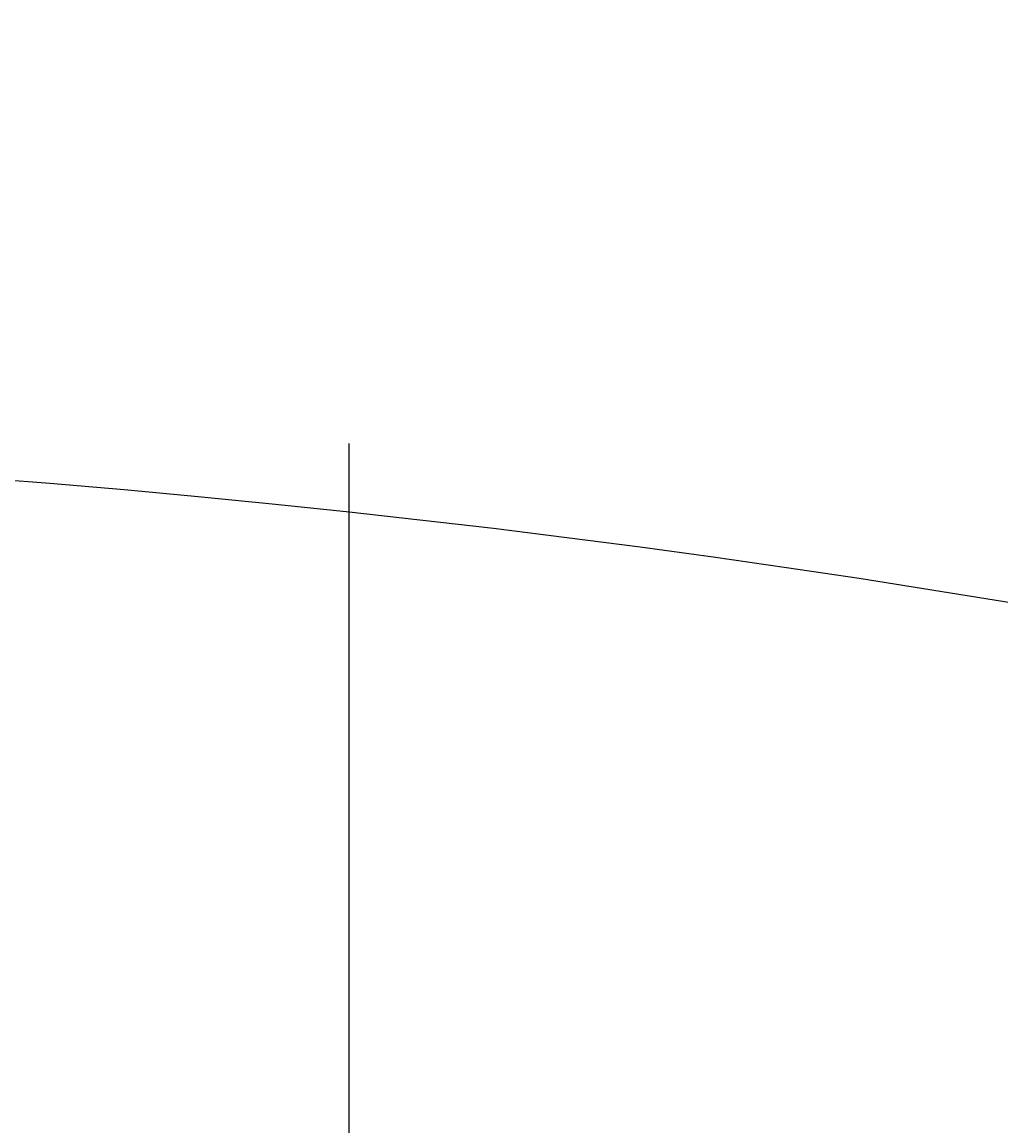
# Model space of a CAD drawing. Units: millimetres. Extents: x 19292 to 100733, y 12374 to 26974.
# Tile 10 of 24: x 29528 to 29589, y 15599 to 15668. Entities that reach past the tile are written whole.
import ezdxf

# ---------------------------------------------------------------- set-up
doc = ezdxf.new("R2010")
doc.units = ezdxf.units.MM
doc.layers.add('A-ANNO-DIMS', color=2, linetype='Continuous', lineweight=18)
doc.layers.add('A-DOOR', color=4, linetype='Continuous', lineweight=25)
doc.styles.get("Standard").update_dxf_attribs({"font": 'arial.ttf'})
doc.dimstyles.get("Standard").update_dxf_attribs({"dimtxt": 0.18, "dimasz": 0.18, "dimexe": 0.18, "dimexo": 0.0625, "dimgap": 0.09, "dimtad": 0, "dimtih": 1, "dimtoh": 1, "dimdec": 4, "dimzin": 0, "dimdsep": 46, "dimtxsty": 'Standard', "dimcen": 0.09, "dimadec": 0, "dimazin": 0, "dimtfac": 1, "dimtdec": 4, "dimtofl": 0, "dimtmove": 0, "dimatfit": 3, "dimfxl": 1, "dimtolj": 1, "dimtzin": 0, "dimarcsym": 0})

# ---------------------------------------------------------------- blocks, each defined once
blk = doc.blocks.new('*D79')
at = {"layer": 'A-ANNO-DIMS', "color": 0, "lineweight": -2, "transparency": 16777216}
for p, q in [((22694.132, 22860.662), (22694.132, 12808.813)), ((36144.169, 15985.662), (36144.169, 12808.813)), ((22694.312, 12808.993), (29418.731, 12808.993)), ((36143.989, 12808.993), (29419.571, 12808.993))]:
    blk.add_line(p, q, dxfattribs=at)
at = {"layer": 'A-ANNO-DIMS', "color": 0, "transparency": 16777216}
for points in [[(22694.312, 12809.023), (22694.312, 12808.963), (22694.132, 12808.993)], [(36143.989, 12809.023), (36143.989, 12808.963), (36144.169, 12808.993)]]:
    blk.add_solid(points, dxfattribs=at)
at = {"layer": 'Defpoints', "color": 0, "transparency": 16777216}
for p in [(22694.132, 22860.725), (36144.169, 15985.725), (36144.169, 12808.993)]:
    blk.add_point(p, dxfattribs=at)
at = {"layer": 'A-ANNO-DIMS', "color": 0, "transparency": 16777216, "insert": (29419.151, 12808.993), "char_height": 0.18, "attachment_point": 5}
blk.add_mtext('\\A1;13450', dxfattribs=at)
blk = doc.blocks.new('*D82')
at = {"layer": 'A-ANNO-DIMS', "color": 0, "lineweight": -2, "transparency": 16777216}
for p, q in [((27198.815, 13562.81), (27198.815, 23555.905)), ((27198.995, 23555.725), (29296.444, 23555.725)), ((31394.619, 23555.725), (29297.169, 23555.725)), ((31394.799, 13544.055), (31394.799, 23555.905))]:
    blk.add_line(p, q, dxfattribs=at)
at = {"layer": 'A-ANNO-DIMS', "color": 0, "transparency": 16777216}
for points in [[(27198.995, 23555.755), (27198.995, 23555.695), (27198.815, 23555.725)], [(31394.619, 23555.755), (31394.619, 23555.695), (31394.799, 23555.725)]]:
    blk.add_solid(points, dxfattribs=at)
at = {"layer": 'Defpoints', "color": 0, "transparency": 16777216}
for p in [(31394.799, 23555.725), (27198.815, 13562.748), (31394.799, 13543.993)]:
    blk.add_point(p, dxfattribs=at)
at = {"layer": 'A-ANNO-DIMS', "color": 0, "transparency": 16777216, "insert": (29296.807, 23555.725), "char_height": 0.18, "attachment_point": 5}
blk.add_mtext('\\A1;4196', dxfattribs=at)
blk = doc.blocks.new('*D86')
at = {"layer": 'A-ANNO-DIMS', "color": 0, "lineweight": -2, "transparency": 16777216}
for p, q in [((27198.815, 15132.81), (27198.815, 23555.905)), ((27198.995, 23555.725), (29198.453, 23555.725)), ((31198.635, 23555.725), (29199.177, 23555.725)), ((31198.815, 15132.81), (31198.815, 23555.905))]:
    blk.add_line(p, q, dxfattribs=at)
at = {"layer": 'A-ANNO-DIMS', "color": 0, "transparency": 16777216}
for points in [[(27198.995, 23555.755), (27198.995, 23555.695), (27198.815, 23555.725)], [(31198.635, 23555.755), (31198.635, 23555.695), (31198.815, 23555.725)]]:
    blk.add_solid(points, dxfattribs=at)
at = {"layer": 'Defpoints', "color": 0, "transparency": 16777216}
for p in [(31198.815, 23555.725), (27198.815, 15132.748), (31198.815, 15132.748)]:
    blk.add_point(p, dxfattribs=at)
at = {"layer": 'A-ANNO-DIMS', "color": 0, "transparency": 16777216, "insert": (29198.815, 23555.725), "char_height": 0.18, "attachment_point": 5}
blk.add_mtext('\\A1;4000', dxfattribs=at)

msp = doc.modelspace()

# ---------------------------------------------------------------- linework, layer by layer
at = {"layer": 'A-DOOR'}
msp.add_line((29548.571, 14906.403), (29548.571, 15641.675), dxfattribs=at)
msp.add_arc((29468.571, 14906.403), 735.272, 0, 90, dxfattribs=at)

# ---------------------------------------------------------------- dimensions: what is measured, and where the dimension line sits
at = {"layer": 'A-ANNO-DIMS'}
for base, p1, p2, picture, middle in [((31394.799, 23555.725), (27198.815, 13562.748), (31394.799, 13543.993), '*D82', (29296.807, 23555.725)), ((31198.815, 23555.725), (27198.815, 15132.748), (31198.815, 15132.748), '*D86', (29198.815, 23555.725)), ((36144.169, 12808.993), (22694.132, 22860.725), (36144.169, 15985.725), '*D79', (29419.151, 12808.993))]:
    dim = msp.add_linear_dim(base=base, p1=p1, p2=p2, dimstyle='Standard', override={"dimdec": 0, "dimlfac": 1, "dimrnd": 0, "dimzin": 0, "dimdsep": 46, "dimlunit": 2}, dxfattribs=at)
    dim.commit()
    dim.dimension.update_dxf_attribs({"geometry": picture, "text_midpoint": middle})

doc.saveas('drawing.dxf')
